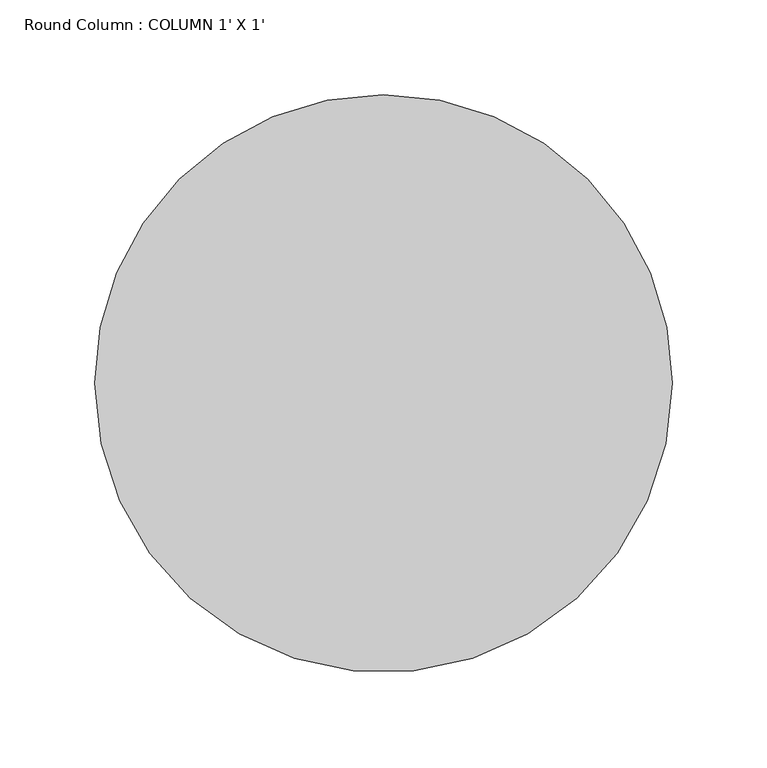
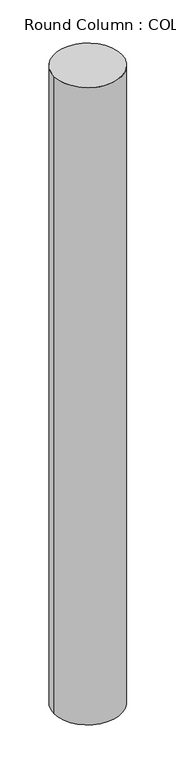
"""IFC4 building model written with IfcOpenShell, lengths in millimetres: column geometry, Round Column : COLUMN 1' X 1'."""

from ifc_helpers import new_model, si_unit, point, frame, origin, origin_2d, place, context, project, spatial, circle_curve, trimmed, segment, composite_curve, outline, extrude, source, transform, mapped, element, save


def round_column_column_1_x_1_faae7945(model_context):
    return source(origin(), model_context, "Body", "SweptSolid", [
        extrude(outline(composite_curve([segment(trimmed(circle_curve(origin_2d(), 152.4), [point((152.4, 0.0))], [point((-152.4, 0.0))], False, "CARTESIAN"), True, "CONTINUOUS"), segment(trimmed(circle_curve(origin_2d(), 152.4), [point((-152.4, 0.0))], [point((0.0, 152.4))], False, "CARTESIAN"), True, "CONTINUOUS"), segment(trimmed(circle_curve(origin_2d(), 152.4), [point((0.0, 152.4))], [point((152.4, 0.0))], False, "CARTESIAN"), True, "CONTINUOUS")], self_intersect=False)), frame((0.0, 0.0, 6400.8), z_axis=(0.0, 0.0, 1.0), x_axis=(1.0, 0.0, 0.0)), (0.0, 0.0, 1.0), 3048.0),
    ])


if __name__ == "__main__":
    model = new_model("IFC4")
    model_context = context("Model", 3, world=origin())
    ifc_project = project(units=[si_unit("LENGTHUNIT", "METRE", prefix="MILLI")], contexts=[model_context])
    site = spatial("IfcSite", under=ifc_project)
    building = spatial("IfcBuilding", under=site)
    placement = place(None, origin())
    round_column_column_1_x_1_shape = round_column_column_1_x_1_faae7945(model_context)
    element("IfcColumn", 1, ObjectType="Round Column : COLUMN 1' X 1'", at=placement, inside=building, context=model_context, shape_type="MappedRepresentation", body=[
        mapped(round_column_column_1_x_1_shape, transform((0.0, 0.0, 0.0), x_axis=(1.0, 0.0, 0.0), y_axis=(0.0, 1.0, 0.0), z_axis=(0.0, 0.0, 1.0))),
    ])
    save(model, "model.ifc")

# Revit data of these elements
# Type "Round Column : COLUMN 1' X 1'"
#   Assembly Code = "B1010200"
#   Diameter = 1' - 0"
#   Offset Base = 0' - 0"
#   Offset Top = 0' - 0"
#   Material = CREAM BEIGE COLOUR
# Element 1 (IfcColumn, "Round Column : COLUMN 1' X 1'")
#   Materials on its faces: "CREAM BEIGE COLOUR"
# Materials
#   "CREAM BEIGE COLOUR": class "Generic", colour RGB 120 120 120, transparency 0, Cost = 0
